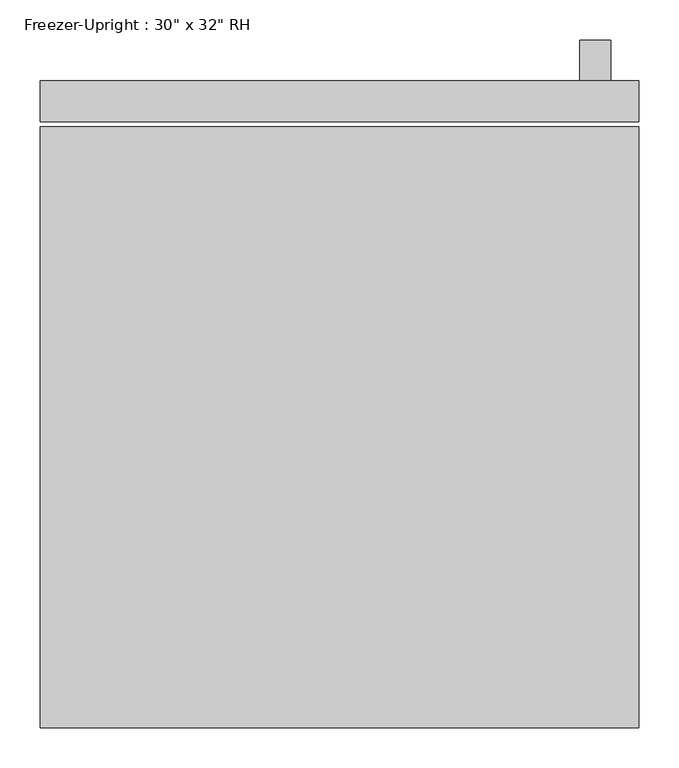
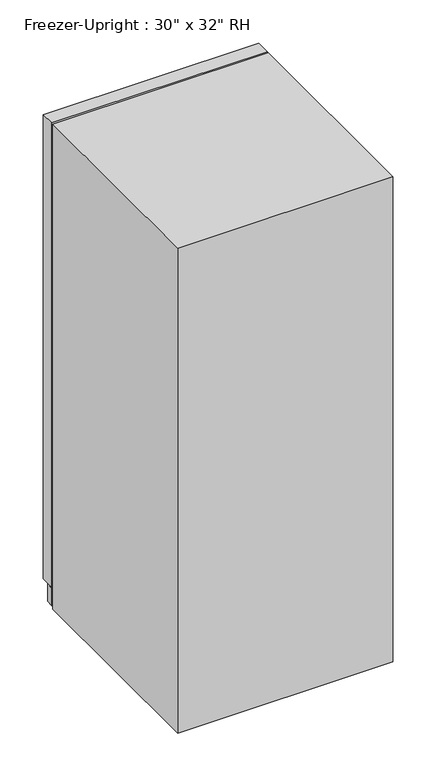
"""IFC4 building model written with IfcOpenShell, lengths in millimetres: proxy geometry."""

from ifc_helpers import new_model, si_unit, frame, origin, origin_with_axes, place, context, project, spatial, polyline, outline, extrude, source, transform, mapped, element, save


def proxy_1d9d56c6(model_context):
    return source(origin(), model_context, "Body", "SweptSolid", [
        extrude(outline(polyline([(373.0625, -388.5489715), (-373.0625, -388.5489715), (-373.0625, 360.7510285), (373.0625, 360.7510285), (373.0625, -388.5489715)])), origin_with_axes(), (0.0, 0.0, 1.0), 1778.0),
        extrude(outline(polyline([(373.0625, 367.1010285), (-373.0625, 367.1010285), (-373.0625, 417.9010285), (373.0625, 417.9010285), (373.0625, 367.1010285)])), frame((0.0, 0.0, 76.2), z_axis=(0.0, 0.0, 1.0), x_axis=(1.0, 0.0, 0.0)), (0.0, 0.0, 1.0), 1701.8),
        extrude(outline(polyline([(373.0625, 367.1010285), (-373.0625, 367.1010285), (-373.0625, 392.5010285), (373.0625, 392.5010285), (373.0625, 367.1010285)])), frame((0.0, 0.0, 9.3816357), z_axis=(0.0, 0.0, 1.0), x_axis=(1.0, 0.0, 0.0)), (0.0, 0.0, 1.0), 63.5),
        extrude(outline(polyline([(417.9010285, 1517.65), (417.9010285, 1524.0), (468.7010285, 1524.0), (468.7010285, 1206.5154683), (417.9010285, 1206.5154683), (417.9010285, 1212.85), (462.3510285, 1212.85), (462.3510285, 1517.65), (417.9010285, 1517.65)])), frame((300.0375, 0.0, 0.0), z_axis=(1.0, 0.0, 0.0), x_axis=(0.0, 1.0, 0.0)), (0.0, 0.0, 1.0), 38.1),
    ])


if __name__ == "__main__":
    model = new_model("IFC4")
    model_context = context("Model", 3, world=origin())
    ifc_project = project(units=[si_unit("LENGTHUNIT", "METRE", prefix="MILLI")], contexts=[model_context])
    site = spatial("IfcSite", under=ifc_project)
    building = spatial("IfcBuilding", under=site)
    placement = place(None, origin())
    proxy_shape = proxy_1d9d56c6(model_context)
    element("IfcBuildingElementProxy", 1, Name="Freezer-Upright : 30\" x 32\" RH", ObjectType="Freezer-Upright : 30\" x 32\" RH", at=placement, inside=building, context=model_context, shape_type="MappedRepresentation", body=[
        mapped(proxy_shape, transform((0.0, 0.0, 0.0), x_axis=(1.0, 0.0, 0.0), y_axis=(0.0, 1.0, 0.0), z_axis=(0.0, 0.0, 1.0))),
    ])
    save(model, "model.ifc")

# Revit data of these elements
# Type "Freezer-Upright : 30\" x 32\" RH"
#   Assembly Code = "E1090400"
#   Depth = 2' - 7 3/4"
#   Handle = 2' - 2 1/2"
#   Height = 5' - 10"
#   Rear Clearance = 0' - 2"
#   Width = 2' - 5 3/8"
#   Material = Metal - Paint Finish - Ivory,Glossy
#   Default Elevation = 0
# Element 1 (IfcBuildingElementProxy, "Freezer-Upright : 30\" x 32\" RH")
#   Materials on its faces: "Metal - Paint Finish - Ivory,Glossy", "Metal - Chrome", "Metal - Paint Finish - Black,Glossy"
# Materials
#   "Metal - Paint Finish - Ivory,Glossy": colour RGB 247 247 239, transparency 0
#   "Metal - Chrome": colour RGB 177 177 177, transparency 0
#   "Metal - Paint Finish - Black,Glossy": colour RGB 0 0 0, transparency 0
